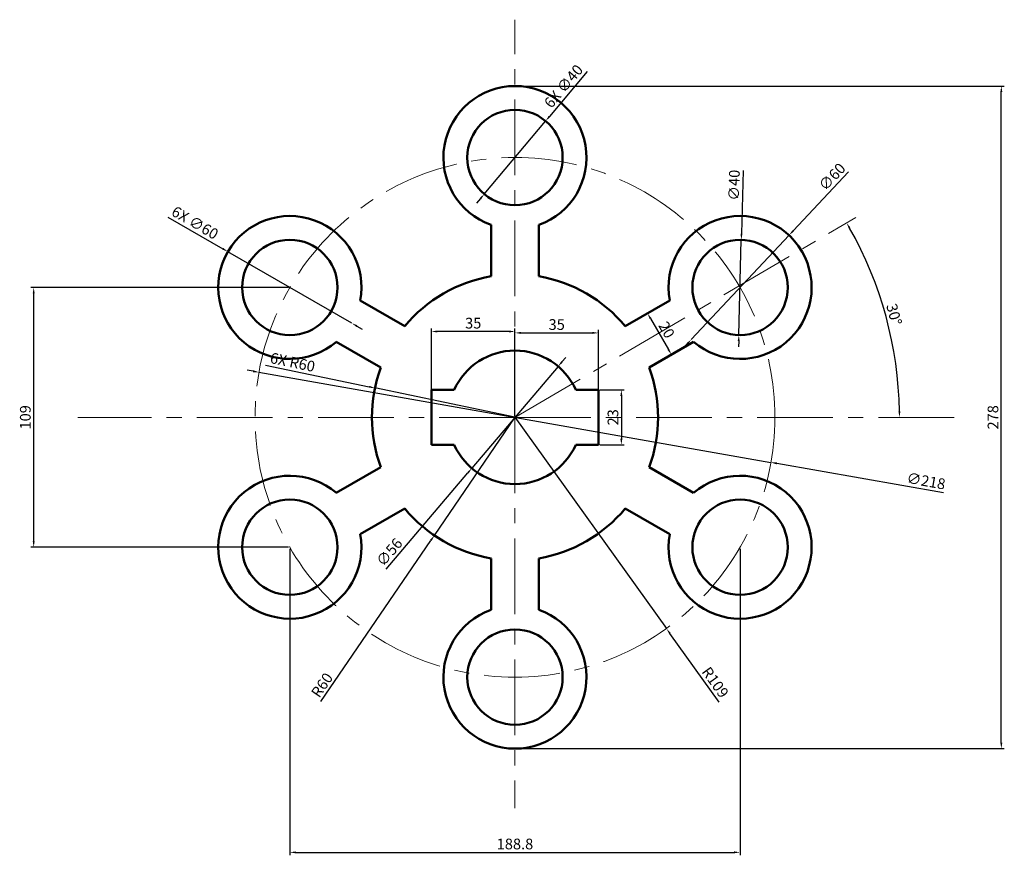
# Model space of a CAD drawing. Units: millimetres. Extents: x 3171 to 3584, y 1424 to 1775.
import ezdxf

# ---------------------------------------------------------------- set-up
doc = ezdxf.new("R2010")
doc.units = ezdxf.units.MM
doc.linetypes.add('CENTER', pattern=[50.8, 31.75, -6.35, 6.35, -6.35])
for name, color, linetype, lineweight in [('M-CNTR', 1, 'CENTER', 18), ('M-DIMS', 120, 'Continuous', 25), ('M-OUTL', 7, 'Continuous', 50)]:
    doc.layers.add(name, color=color, linetype=linetype, lineweight=lineweight)
doc.styles.get("Standard").update_dxf_attribs({"font": 'arial.ttf'})
doc.dimstyles.new('ISO-25', dxfattribs={"dimtxt": 4.5, "dimasz": 2.5, "dimexe": 1.25, "dimexo": 0.625, "dimtad": 1, "dimtxsty": 'Standard', "dimcen": 2.5, "dimadec": 0, "dimazin": 0, "dimtfac": 1, "dimtmove": 0, "dimatfit": 3, "dimfxl": 1, "dimarcsym": 0})

# ---------------------------------------------------------------- blocks, each defined once
blk = doc.blocks.new('*D1')
at = {"layer": 'Defpoints', "color": 0, "transparency": 16777216}
for p in [(3343.56, 1644.25), (3343.56, 1608.24), (3378.56, 1608.24)]:
    blk.add_point(p, dxfattribs=at)
at = {"layer": 'M-DIMS', "color": 0, "lineweight": -2, "transparency": 16777216}
for p, q in [((3343.56, 1608.86), (3343.56, 1645.5)), ((3376.06, 1644.25), (3346.06, 1644.25)), ((3378.56, 1608.86), (3378.56, 1645.5))]:
    blk.add_line(p, q, dxfattribs=at)
at = {"layer": 'M-DIMS', "color": 0, "transparency": 16777216}
for points in [[(3346.06, 1644.67), (3346.06, 1643.83), (3343.56, 1644.25)], [(3376.06, 1644.67), (3376.06, 1643.83), (3378.56, 1644.25)]]:
    blk.add_solid(points, dxfattribs=at)
at = {"layer": 'M-DIMS', "color": 0, "transparency": 16777216, "insert": (3361.06, 1647.17), "char_height": 4.5, "attachment_point": 5}
blk.add_mtext('35', dxfattribs=at)
blk = doc.blocks.new('*D2')
at = {"layer": 'Defpoints', "color": 0, "transparency": 16777216}
for p in [(3413.56, 1643.66), (3378.56, 1608.24), (3413.56, 1608.24)]:
    blk.add_point(p, dxfattribs=at)
at = {"layer": 'M-DIMS', "color": 0, "lineweight": -2, "transparency": 16777216}
for p, q in [((3378.56, 1608.86), (3378.56, 1644.91)), ((3381.06, 1643.66), (3411.06, 1643.66)), ((3413.56, 1608.86), (3413.56, 1644.91))]:
    blk.add_line(p, q, dxfattribs=at)
at = {"layer": 'M-DIMS', "color": 0, "transparency": 16777216}
for points in [[(3381.06, 1644.08), (3381.06, 1643.25), (3378.56, 1643.66)], [(3411.06, 1644.08), (3411.06, 1643.25), (3413.56, 1643.66)]]:
    blk.add_solid(points, dxfattribs=at)
at = {"layer": 'M-DIMS', "color": 0, "transparency": 16777216, "insert": (3396.06, 1646.59), "char_height": 4.5, "attachment_point": 5}
blk.add_mtext('35', dxfattribs=at)
blk = doc.blocks.new('*D3')
at = {"layer": 'Defpoints', "color": 0, "transparency": 16777216}
for p in [(3413.56, 1619.74), (3413.56, 1596.74), (3423.17, 1596.74)]:
    blk.add_point(p, dxfattribs=at)
at = {"layer": 'M-DIMS', "color": 0, "lineweight": -2, "transparency": 16777216}
for p, q in [((3414.19, 1619.74), (3424.42, 1619.74)), ((3423.17, 1617.24), (3423.17, 1599.24)), ((3414.19, 1596.74), (3424.42, 1596.74))]:
    blk.add_line(p, q, dxfattribs=at)
at = {"layer": 'M-DIMS', "color": 0, "transparency": 16777216}
for points in [[(3422.75, 1617.24), (3423.59, 1617.24), (3423.17, 1619.74)], [(3422.75, 1599.24), (3423.59, 1599.24), (3423.17, 1596.74)]]:
    blk.add_solid(points, dxfattribs=at)
at = {"layer": 'M-DIMS', "color": 0, "transparency": 16777216, "insert": (3420.24, 1608.24), "char_height": 4.5, "attachment_point": 5, "rotation": 90}
blk.add_mtext('23', dxfattribs=at)
blk = doc.blocks.new('*D4')
at = {"layer": 'Defpoints', "color": 0, "transparency": 16777216}
for p in [(3434.13, 1651.87), (3444.13, 1634.55), (3444.14, 1634.55)]:
    blk.add_point(p, dxfattribs=at)
at = {"layer": 'M-DIMS', "color": 0, "lineweight": -2, "transparency": 16777216}
for p, q in [((3434.67, 1652.18), (3435.22, 1652.5)), ((3435.39, 1649.71), (3442.89, 1636.72)), ((3444.67, 1634.86), (3445.22, 1635.18))]:
    blk.add_line(p, q, dxfattribs=at)
at = {"layer": 'M-DIMS', "color": 0, "transparency": 16777216}
for points in [[(3435.75, 1649.91), (3435.03, 1649.5), (3434.14, 1651.87)], [(3443.25, 1636.92), (3442.53, 1636.51), (3444.14, 1634.55)]]:
    blk.add_solid(points, dxfattribs=at)
at = {"layer": 'M-DIMS', "color": 0, "transparency": 16777216, "insert": (3441.67, 1644.67), "char_height": 4.5, "attachment_point": 5, "rotation": 300}
blk.add_mtext('20', dxfattribs=at)
blk = doc.blocks.new('*D5')
at = {"layer": 'Defpoints', "color": 0, "transparency": 16777216}
for p in [(3521.53, 1692.08), (3537.28, 1636.6), (3378.56, 1608.24), (3378.56, 1608.24), (3563.95, 1608.24)]:
    blk.add_point(p, dxfattribs=at)
at = {"layer": 'M-DIMS', "color": 0, "lineweight": -2, "transparency": 16777216}
blk.add_arc((3378.56, 1608.24), 161.23, 0.8884, 29.5022, dxfattribs=at)
at = {"layer": 'M-DIMS', "color": 0, "transparency": 16777216}
for points in [[(3518.53, 1687.43), (3519.25, 1687.84), (3517.64, 1689.8)], [(3540.19, 1610.74), (3539.36, 1610.73), (3539.79, 1608.24)]]:
    blk.add_solid(points, dxfattribs=at)
at = {"layer": 'M-DIMS', "color": 0, "transparency": 16777216, "insert": (3536.98, 1651.26), "char_height": 4.5, "attachment_point": 5, "rotation": 285.1953}
blk.add_mtext('30°', dxfattribs=at)
blk = doc.blocks.new('*D6')
at = {"layer": 'Defpoints', "color": 0, "transparency": 16777216}
for p in [(3378.56, 1608.24), (3442.06, 1519.64)]:
    blk.add_point(p, dxfattribs=at)
at = {"layer": 'M-DIMS', "color": 0, "lineweight": -2, "transparency": 16777216}
for p, q in [((3378.56, 1608.24), (3442.06, 1519.64)), ((3464.23, 1488.7), (3443.52, 1517.61))]:
    blk.add_line(p, q, dxfattribs=at)
at = {"layer": 'M-DIMS', "color": 0, "transparency": 16777216}
blk.add_solid([(3443.85, 1517.85), (3443.18, 1517.37), (3442.06, 1519.64)], dxfattribs=at)
at = {"layer": 'M-DIMS', "color": 0, "transparency": 16777216, "insert": (3462.09, 1496.71), "char_height": 4.5, "attachment_point": 5, "rotation": 305.6286}
blk.add_mtext('R109', dxfattribs=at)
blk = doc.blocks.new('*D7')
at = {"layer": 'Defpoints', "color": 0, "transparency": 16777216}
for p in [(3378.56, 1608.24), (3344.74, 1558.68)]:
    blk.add_point(p, dxfattribs=at)
at = {"layer": 'M-DIMS', "color": 0, "lineweight": -2, "transparency": 16777216}
for p, q in [((3378.56, 1608.24), (3344.74, 1558.68)), ((3297.18, 1488.97), (3343.33, 1556.61))]:
    blk.add_line(p, q, dxfattribs=at)
at = {"layer": 'M-DIMS', "color": 0, "transparency": 16777216}
blk.add_solid([(3342.99, 1556.85), (3343.68, 1556.38), (3344.74, 1558.68)], dxfattribs=at)
at = {"layer": 'M-DIMS', "color": 0, "transparency": 16777216, "insert": (3298.14, 1495.57), "char_height": 4.5, "attachment_point": 5, "rotation": 55.6897}
blk.add_mtext('R60', dxfattribs=at)
blk = doc.blocks.new('*D8')
at = {"layer": 'Defpoints', "color": 0, "transparency": 16777216}
for p in [(3396.67, 1629.6), (3360.46, 1586.88)]:
    blk.add_point(p, dxfattribs=at)
at = {"layer": 'M-DIMS', "color": 0, "lineweight": -2, "transparency": 16777216}
for p, q in [((3398.28, 1631.51), (3399.9, 1633.41)), ((3396.67, 1629.6), (3360.46, 1586.88)), ((3324.57, 1544.53), (3358.85, 1584.97))]:
    blk.add_line(p, q, dxfattribs=at)
at = {"layer": 'M-DIMS', "color": 0, "transparency": 16777216}
for points in [[(3397.97, 1631.77), (3398.6, 1631.24), (3396.67, 1629.6)], [(3358.53, 1585.24), (3359.16, 1584.7), (3360.46, 1586.88)]]:
    blk.add_solid(points, dxfattribs=at)
at = {"layer": 'M-DIMS', "color": 0, "transparency": 16777216, "insert": (3326.32, 1551.3), "char_height": 4.5, "attachment_point": 5, "rotation": 49.7194}
blk.add_mtext('∅56', dxfattribs=at)
blk = doc.blocks.new('*D9')
at = {"layer": 'Defpoints', "color": 0, "transparency": 16777216}
for p in [(3493.48, 1684.62), (3452.44, 1640.85)]:
    blk.add_point(p, dxfattribs=at)
at = {"layer": 'M-DIMS', "color": 0, "lineweight": -2, "transparency": 16777216}
for p, q in [((3518.47, 1711.27), (3495.19, 1686.45)), ((3452.44, 1640.85), (3493.48, 1684.62)), ((3450.73, 1639.03), (3449.02, 1637.21))]:
    blk.add_line(p, q, dxfattribs=at)
at = {"layer": 'M-DIMS', "color": 0, "transparency": 16777216}
for points in [[(3494.89, 1686.73), (3495.5, 1686.16), (3493.48, 1684.62)], [(3450.43, 1639.31), (3451.03, 1638.74), (3452.44, 1640.85)]]:
    blk.add_solid(points, dxfattribs=at)
at = {"layer": 'M-DIMS', "color": 0, "transparency": 16777216, "insert": (3511.94, 1708.77), "char_height": 4.5, "attachment_point": 5, "rotation": 46.8429}
blk.add_mtext('∅60', dxfattribs=at)
blk = doc.blocks.new('*D10')
at = {"layer": 'Defpoints', "color": 0, "transparency": 16777216}
for p in [(3473.48, 1682.73), (3472.44, 1642.74)]:
    blk.add_point(p, dxfattribs=at)
at = {"layer": 'M-DIMS', "color": 0, "lineweight": -2, "transparency": 16777216}
for p, q in [((3474.24, 1711.83), (3473.54, 1685.23)), ((3472.44, 1642.74), (3473.48, 1682.73)), ((3472.38, 1640.25), (3472.31, 1637.75))]:
    blk.add_line(p, q, dxfattribs=at)
at = {"layer": 'M-DIMS', "color": 0, "transparency": 16777216}
for points in [[(3473.13, 1685.24), (3473.96, 1685.22), (3473.48, 1682.73)], [(3471.96, 1640.26), (3472.79, 1640.23), (3472.44, 1642.74)]]:
    blk.add_solid(points, dxfattribs=at)
at = {"layer": 'M-DIMS', "color": 0, "transparency": 16777216, "insert": (3471.02, 1705.63), "char_height": 4.5, "attachment_point": 5, "rotation": 88.5134}
blk.add_mtext('∅40', dxfattribs=at)
blk = doc.blocks.new('SPIDER-ARM-D60-BORE40')
for p, q in [((-10, -28.28), (-10, -49.84)), ((10, -28.28), (10, -49.84))]:
    blk.add_line(p, q)
blk.add_circle((0, 0), 20)
blk.add_arc((0, 0), 30, 289.4712, 250.5288)
blk = doc.blocks.new('*D12')
at = {"layer": 'Defpoints', "color": 0, "transparency": 16777216}
for p in [(3284.17, 1553.74), (3472.96, 1553.74), (3472.96, 1425.73)]:
    blk.add_point(p, dxfattribs=at)
at = {"layer": 'M-DIMS', "color": 0, "lineweight": -2, "transparency": 16777216}
for p, q in [((3284.17, 1553.11), (3284.17, 1424.48)), ((3472.96, 1553.11), (3472.96, 1424.48)), ((3286.67, 1425.73), (3470.46, 1425.73))]:
    blk.add_line(p, q, dxfattribs=at)
at = {"layer": 'M-DIMS', "color": 0, "transparency": 16777216}
for points in [[(3286.67, 1426.15), (3286.67, 1425.31), (3284.17, 1425.73)], [(3470.46, 1426.15), (3470.46, 1425.31), (3472.96, 1425.73)]]:
    blk.add_solid(points, dxfattribs=at)
at = {"layer": 'M-DIMS', "color": 0, "transparency": 16777216, "insert": (3378.56, 1428.65), "char_height": 4.5, "attachment_point": 5}
blk.add_mtext('188.8', dxfattribs=at)
blk = doc.blocks.new('*D13')
at = {"layer": 'Defpoints', "color": 0, "transparency": 16777216}
for p in [(3378.56, 1747.24), (3582.5, 1747.24), (3378.56, 1469.24)]:
    blk.add_point(p, dxfattribs=at)
at = {"layer": 'M-DIMS', "color": 0, "lineweight": -2, "transparency": 16777216}
for p, q in [((3379.19, 1747.24), (3583.75, 1747.24)), ((3582.5, 1471.74), (3582.5, 1744.74)), ((3379.19, 1469.24), (3583.75, 1469.24))]:
    blk.add_line(p, q, dxfattribs=at)
at = {"layer": 'M-DIMS', "color": 0, "transparency": 16777216}
for points in [[(3582.08, 1744.74), (3582.91, 1744.74), (3582.5, 1747.24)], [(3582.08, 1471.74), (3582.91, 1471.74), (3582.5, 1469.24)]]:
    blk.add_solid(points, dxfattribs=at)
at = {"layer": 'M-DIMS', "color": 0, "transparency": 16777216, "insert": (3579.58, 1608.24), "char_height": 4.5, "attachment_point": 5, "rotation": 90}
blk.add_mtext('278', dxfattribs=at)
blk = doc.blocks.new('*D14')
at = {"layer": 'Defpoints', "color": 0, "transparency": 16777216}
for p in [(3176.77, 1662.74), (3284.17, 1662.74), (3284.17, 1553.74)]:
    blk.add_point(p, dxfattribs=at)
at = {"layer": 'M-DIMS', "color": 0, "lineweight": -2, "transparency": 16777216}
for p, q in [((3283.54, 1662.74), (3175.52, 1662.74)), ((3176.77, 1556.24), (3176.77, 1660.24)), ((3283.54, 1553.74), (3175.52, 1553.74))]:
    blk.add_line(p, q, dxfattribs=at)
at = {"layer": 'M-DIMS', "color": 0, "transparency": 16777216}
for points in [[(3176.35, 1660.24), (3177.18, 1660.24), (3176.77, 1662.74)], [(3176.35, 1556.24), (3177.18, 1556.24), (3176.77, 1553.74)]]:
    blk.add_solid(points, dxfattribs=at)
at = {"layer": 'M-DIMS', "color": 0, "transparency": 16777216, "insert": (3173.84, 1608.24), "char_height": 4.5, "attachment_point": 5, "rotation": 90}
blk.add_mtext('109', dxfattribs=at)
blk = doc.blocks.new('*D15')
at = {"layer": 'Defpoints', "color": 0, "transparency": 16777216}
for p in [(3271.22, 1627.16), (3485.91, 1589.31)]:
    blk.add_point(p, dxfattribs=at)
at = {"layer": 'M-DIMS', "color": 0, "lineweight": -2, "transparency": 16777216}
for p, q in [((3268.76, 1627.6), (3266.3, 1628.03)), ((3271.22, 1627.16), (3485.91, 1589.31)), ((3558.24, 1576.56), (3488.37, 1588.88))]:
    blk.add_line(p, q, dxfattribs=at)
at = {"layer": 'M-DIMS', "color": 0, "transparency": 16777216}
for points in [[(3268.83, 1628.01), (3268.69, 1627.19), (3271.22, 1627.16)], [(3488.44, 1589.29), (3488.3, 1588.47), (3485.91, 1589.31)]]:
    blk.add_solid(points, dxfattribs=at)
at = {"layer": 'M-DIMS', "color": 0, "transparency": 16777216, "insert": (3550.84, 1580.96), "char_height": 4.5, "attachment_point": 5, "rotation": 350.0003}
blk.add_mtext('∅218', dxfattribs=at)
blk = doc.blocks.new('*D16')
at = {"layer": 'Defpoints', "color": 0, "transparency": 16777216}
for p in [(3258.19, 1677.74), (3310.15, 1647.74)]:
    blk.add_point(p, dxfattribs=at)
at = {"layer": 'M-DIMS', "color": 0, "lineweight": -2, "transparency": 16777216}
for p, q in [((3233.06, 1692.24), (3256.02, 1678.99)), ((3310.15, 1647.74), (3258.19, 1677.74)), ((3312.31, 1646.49), (3314.48, 1645.24))]:
    blk.add_line(p, q, dxfattribs=at)
at = {"layer": 'M-DIMS', "color": 0, "transparency": 16777216}
for points in [[(3256.23, 1679.35), (3255.81, 1678.63), (3258.19, 1677.74)], [(3312.52, 1646.85), (3312.11, 1646.13), (3310.15, 1647.74)]]:
    blk.add_solid(points, dxfattribs=at)
at = {"layer": 'M-DIMS', "color": 0, "transparency": 16777216, "insert": (3244.12, 1689.38), "char_height": 4.5, "attachment_point": 5, "rotation": 330.0005}
blk.add_mtext('6X ∅60', dxfattribs=at)
blk = doc.blocks.new('*D17')
at = {"layer": 'Defpoints', "color": 0, "transparency": 16777216}
for p in [(3391.42, 1732.56), (3365.71, 1701.92)]:
    blk.add_point(p, dxfattribs=at)
at = {"layer": 'M-DIMS', "color": 0, "lineweight": -2, "transparency": 16777216}
for p, q in [((3408.79, 1753.27), (3393.03, 1734.47)), ((3365.71, 1701.92), (3391.42, 1732.56)), ((3364.1, 1700), (3362.5, 1698.09))]:
    blk.add_line(p, q, dxfattribs=at)
at = {"layer": 'M-DIMS', "color": 0, "transparency": 16777216}
for points in [[(3392.71, 1734.74), (3393.35, 1734.21), (3391.42, 1732.56)], [(3363.78, 1700.27), (3364.42, 1699.73), (3365.71, 1701.92)]]:
    blk.add_solid(points, dxfattribs=at)
at = {"layer": 'M-DIMS', "color": 0, "transparency": 16777216, "insert": (3399.38, 1746.79), "char_height": 4.5, "attachment_point": 5, "rotation": 50.0032}
blk.add_mtext('6X ∅40', dxfattribs=at)
blk = doc.blocks.new('*D18')
at = {"layer": 'Defpoints', "color": 0, "transparency": 16777216}
for p in [(3319.84, 1620.55), (3378.56, 1608.24)]:
    blk.add_point(p, dxfattribs=at)
at = {"layer": 'M-DIMS', "color": 0, "lineweight": -2, "transparency": 16777216}
for p, q in [((3274, 1630.16), (3317.39, 1621.06)), ((3378.56, 1608.24), (3319.84, 1620.55))]:
    blk.add_line(p, q, dxfattribs=at)
at = {"layer": 'M-DIMS', "color": 0, "transparency": 16777216}
blk.add_solid([(3317.48, 1621.47), (3317.31, 1620.65), (3319.84, 1620.55)], dxfattribs=at)
at = {"layer": 'M-DIMS', "color": 0, "transparency": 16777216, "insert": (3285.21, 1630.8), "char_height": 4.5, "attachment_point": 5, "rotation": 348.1585}
blk.add_mtext('6X R60', dxfattribs=at)

msp = doc.modelspace()

# ---------------------------------------------------------------- linework, layer by layer
at = {"layer": 'M-CNTR'}
for q in [(3378.564, 1775.077), (3521.527, 1692.082), (3195.317, 1608.237), (3563.948, 1608.237), (3378.564, 1444.279)]:
    msp.add_line((3378.564, 1608.237), q, dxfattribs=at)
msp.add_circle((3378.564, 1608.237), 109, dxfattribs=at)
at = {"layer": 'M-OUTL'}
for p, q in [((3343.564, 1608.237), (3343.564, 1619.737)), ((3343.564, 1619.737), (3353.035, 1619.737)), ((3404.094, 1619.737), (3413.564, 1619.737)), ((3413.564, 1619.737), (3413.564, 1596.737)), ((3343.564, 1596.737), (3343.564, 1608.237)), ((3353.035, 1596.737), (3343.564, 1596.737)), ((3413.564, 1596.737), (3404.094, 1596.737))]:
    msp.add_line(p, q, dxfattribs=at)
for radius, start, end in [(60, 99.59407, 140.40593), (60, 39.59407, 80.40593), (28, 24.24971, 155.75029), (60, 159.59407, 200.40593), (60, 339.59407, 20.40593), (28, 204.24971, 335.75029), (60, 219.59407, 260.40593), (60, 279.59407, 320.40593)]:
    msp.add_arc((3378.564, 1608.237), radius, start, end, dxfattribs=at)

# ---------------------------------------------------------------- block references
msp.add_blockref('SPIDER-ARM-D60-BORE40', (3378.564, 1717.237), dxfattribs=at)
for p, rotation in [((3284.168, 1662.737), 60.0000000000006), ((3472.961, 1662.737), 299.9999999999998), ((3284.168, 1553.737), 120.0000000000013), ((3472.961, 1553.737), 240.0000000000025), ((3378.564, 1499.237), 180)]:
    msp.add_blockref('SPIDER-ARM-D60-BORE40', p, dxfattribs=dict(at, rotation=rotation))

# ---------------------------------------------------------------- dimensions: what is measured, and where the dimension line sits
at = {"layer": 'M-DIMS'}
for p1, p2, picture, middle in [((3365.709, 1701.916), (3391.419, 1732.559), '*D17', (3401.713, 1744.828)), ((3310.148, 1647.738), (3258.187, 1677.737), '*D16', (3242.598, 1686.737))]:
    dim = msp.add_diameter_dim_2p(p1=p1, p2=p2, text='6X <>', dimstyle='ISO-25', override={"dimdec": 0, "dimlfac": 1, "dimrnd": 0, "dimzin": 0, "dimdsep": 46, "dimlunit": 2}, dxfattribs=at)
    dim.commit()
    dim.dimension.update_dxf_attribs({"geometry": picture, "text_midpoint": middle, "dimtype": 163})
for base, p1, p2, override, picture, middle in [((3582.498, 1747.237), (3378.564, 1469.237), (3378.564, 1747.237), {"dimdec": 0, "dimlfac": 1, "dimrnd": 0, "dimzin": 0, "dimdsep": 46, "dimlunit": 2}, '*D13', (3579.575, 1608.237)), ((3176.767, 1662.737), (3284.168, 1553.737), (3284.168, 1662.737), {"dimdec": 0, "dimlfac": 1, "dimrnd": 0, "dimzin": 0, "dimdsep": 46, "dimlunit": 2}, '*D14', (3173.845, 1608.237)), ((3423.168, 1596.737), (3413.564, 1619.737), (3413.564, 1596.737), {"dimclrd": 0, "dimclre": 0, "dimclrt": 0}, '*D3', (3420.244, 1608.237))]:
    dim = msp.add_linear_dim(base=base, p1=p1, p2=p2, angle=90, dimstyle='ISO-25', override=override, dxfattribs=at)
    dim.commit()
    dim.dimension.update_dxf_attribs({"geometry": picture, "text_midpoint": middle})
for p1, p2, override, picture, middle in [((3452.441, 1640.853), (3493.481, 1684.622), {"dimclrd": 0, "dimclre": 0, "dimclrt": 0}, '*D9', (3514.164, 1706.68)), ((3472.442, 1642.744), (3473.48, 1682.731), {"dimclrd": 0, "dimclre": 0, "dimclrt": 0}, '*D10', (3474.072, 1705.549)), ((3396.667, 1629.598), (3360.461, 1586.877), {"dimclrd": 0, "dimclre": 0, "dimclrt": 0}, '*D8', (3328.643, 1549.331)), ((3271.22, 1627.165), (3485.908, 1589.31), {"dimdec": 0, "dimlfac": 1, "dimrnd": 0, "dimzin": 0, "dimdsep": 46, "dimlunit": 2}, '*D15', (3550.315, 1577.954))]:
    dim = msp.add_diameter_dim_2p(p1=p1, p2=p2, dimstyle='ISO-25', override=override, dxfattribs=at)
    dim.commit()
    dim.dimension.update_dxf_attribs({"geometry": picture, "text_midpoint": middle, "dimtype": 163})
dim = msp.add_angular_dim_2l(base=(3537.279, 1636.595), line1=((3378.564, 1608.237), (3563.948, 1608.237)), line2=((3378.564, 1608.237), (3521.527, 1692.082)), dimstyle='ISO-25', override={"dimclrd": 0, "dimclre": 0, "dimclrt": 0}, dxfattribs=at)
dim.commit()
dim.dimension.update_dxf_attribs({"geometry": '*D5', "text_midpoint": (3536.977, 1651.263)})
dim = msp.add_aligned_dim(p1=(3434.133, 1651.867), p2=(3444.133, 1634.546), distance=0.008, dimstyle='ISO-25', override={"dimclrd": 0, "dimclre": 0, "dimclrt": 0}, dxfattribs=at)
dim.commit()
dim.dimension.update_dxf_attribs({"geometry": '*D4', "text_midpoint": (3441.671, 1644.672)})
for base, p1, p2, override, picture, middle in [((3343.564, 1644.251), (3378.564, 1608.237), (3343.564, 1608.237), {"dimclrd": 0, "dimclre": 0, "dimclrt": 0}, '*D1', (3361.064, 1647.175)), ((3413.564, 1643.662), (3378.564, 1608.237), (3413.564, 1608.237), {"dimclrd": 0, "dimclre": 0, "dimclrt": 0}, '*D2', (3396.064, 1646.586)), ((3472.961, 1425.729), (3284.168, 1553.737), (3472.961, 1553.737), {"dimdec": 1, "dimlfac": 1, "dimrnd": 0, "dimzin": 0, "dimdsep": 46, "dimlunit": 2}, '*D12', (3378.564, 1428.652))]:
    dim = msp.add_linear_dim(base=base, p1=p1, p2=p2, dimstyle='ISO-25', override=override, dxfattribs=at)
    dim.commit()
    dim.dimension.update_dxf_attribs({"geometry": picture, "text_midpoint": middle})
dim = msp.add_radius_dim(center=(3378.564, 1608.237), mpoint=(3319.841, 1620.55), text='6X <>', dimstyle='ISO-25', override={"dimdec": 0, "dimlfac": 1, "dimrnd": 0, "dimzin": 0, "dimdsep": 46, "dimlunit": 2}, dxfattribs=at)
dim.commit()
dim.dimension.update_dxf_attribs({"geometry": '*D18', "text_midpoint": (3284.607, 1627.937), "dimtype": 164})
for mpoint, picture, middle in [((3344.744, 1558.678), '*D7', (3300.555, 1493.925)), ((3442.06, 1519.641), '*D6', (3459.717, 1495.004))]:
    dim = msp.add_radius_dim(center=(3378.564, 1608.237), mpoint=mpoint, dimstyle='ISO-25', override={"dimclrd": 0, "dimclre": 0, "dimclrt": 0}, dxfattribs=at)
    dim.commit()
    dim.dimension.update_dxf_attribs({"geometry": picture, "text_midpoint": middle, "dimtype": 164})

doc.saveas('drawing.dxf')
